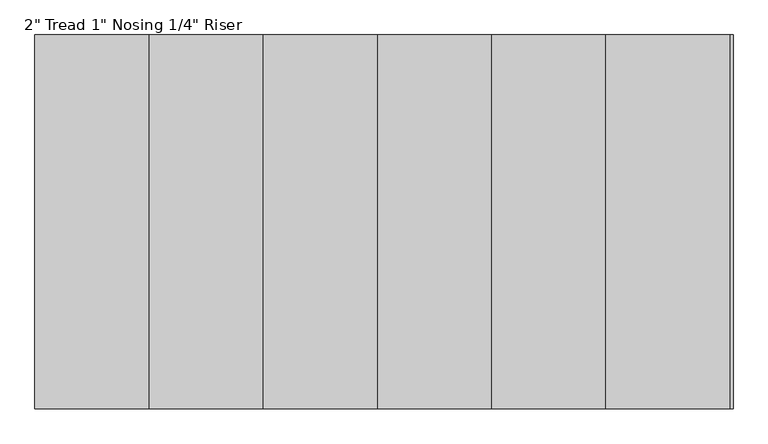
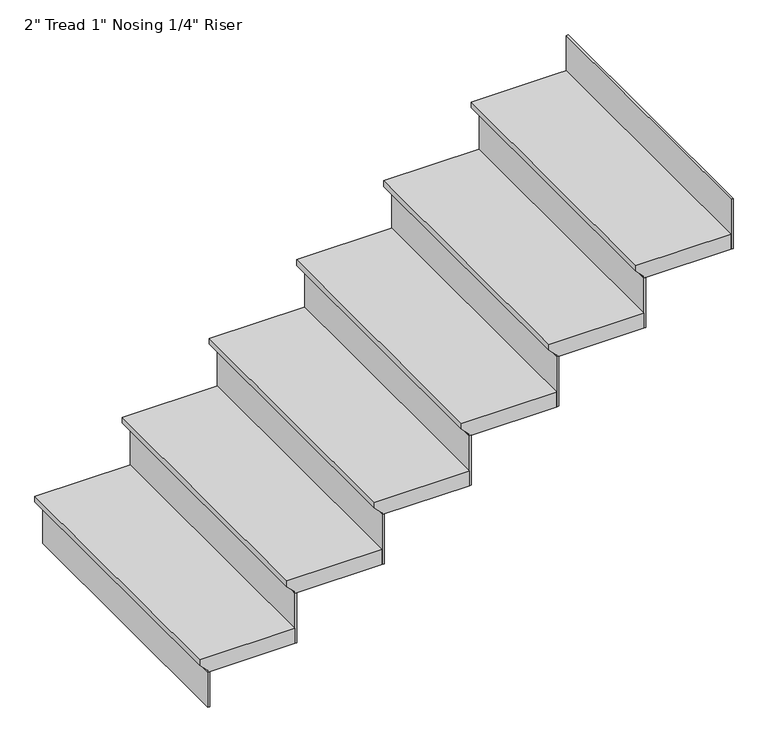
"""IFC4 building model written with IfcOpenShell, lengths in millimetres: stair flight geometry."""

from ifc_helpers import new_model, si_unit, origin, place, context, project, spatial, faceted_brep, source, transform, mapped, element, save


def stair_flight_dd3871da(model_context):
    return source(origin(), model_context, "Body", "Brep", [
        faceted_brep([(-2479.5608498, 3565.3115866, 150.2833333), (-2479.5608498, 3565.3115866, 169.3333333), (-2479.5608498, 4479.7115866, 169.3333333), (-2479.5608498, 4479.7115866, 150.2833333), (-2454.1608498, 3565.3115866, 124.8833333), (-2454.1608498, 4479.7115866, 124.8833333), (-2174.7608498, 3565.3115866, 169.3333333), (-2174.7608498, 4479.7115866, 169.3333333), (-2454.1608498, 4479.7115866, 118.5333333), (-2174.7608498, 4479.7115866, 118.5333333), (-2174.7608498, 3565.3115866, 118.5333333), (-2454.1608498, 3565.3115866, 118.5333333)], [[[0, 1, 2, 3]], [[4, 0, 3, 5]], [[2, 1, 6, 7]], [[8, 9, 10, 11]], [[2, 7, 9, 8, 5, 3]], [[8, 11, 4, 5]], [[6, 1, 0, 4, 11, 10]], [[7, 6, 10, 9]]]),
        faceted_brep([(-2454.1608498, 3565.3115866, 118.5333333), (-2454.1608498, 3565.3115866, 0.0), (-2447.8108498, 3565.3115866, 0.0), (-2447.8108498, 3565.3115866, 118.5333333), (-2454.1608498, 4479.7115866, 118.5333333), (-2447.8108498, 4479.7115866, 118.5333333), (-2447.8108498, 4479.7115866, 0.0), (-2454.1608498, 4479.7115866, 0.0)], [[[0, 1, 2, 3]], [[4, 5, 6, 7]], [[1, 0, 4, 7]], [[2, 1, 7, 6]], [[3, 2, 6, 5]], [[0, 3, 5, 4]]]),
        faceted_brep([(-2174.7608498, 3565.3115866, 287.8666667), (-2174.7608498, 3565.3115866, 118.5333333), (-2168.4108498, 3565.3115866, 118.5333333), (-2168.4108498, 3565.3115866, 287.8666667), (-2174.7608498, 4479.7115866, 287.8666667), (-2168.4108498, 4479.7115866, 287.8666667), (-2168.4108498, 4479.7115866, 118.5333333), (-2174.7608498, 4479.7115866, 118.5333333)], [[[0, 1, 2, 3]], [[4, 5, 6, 7]], [[1, 0, 4, 7]], [[2, 1, 7, 6]], [[3, 2, 6, 5]], [[0, 3, 5, 4]]]),
        faceted_brep([(-2200.1608498, 4479.7115866, 338.6666667), (-2200.1608498, 3565.3115866, 338.6666667), (-1895.3608498, 3565.3115866, 338.6666667), (-1895.3608498, 4479.7115866, 338.6666667), (-2174.7608498, 4479.7115866, 287.8666667), (-1895.3608498, 4479.7115866, 287.8666667), (-1895.3608498, 3565.3115866, 287.8666667), (-2174.7608498, 3565.3115866, 287.8666667), (-2174.7608498, 4479.7115866, 294.2166667), (-2200.1608498, 4479.7115866, 319.6166667), (-2174.7608498, 3565.3115866, 294.2166667), (-2200.1608498, 3565.3115866, 319.6166667)], [[[0, 1, 2, 3]], [[4, 5, 6, 7]], [[0, 3, 5, 4, 8, 9]], [[4, 7, 10, 8]], [[2, 1, 11, 10, 7, 6]], [[3, 2, 6, 5]], [[11, 1, 0, 9]], [[10, 11, 9, 8]]]),
        faceted_brep([(-1895.3608498, 3565.3115866, 457.2), (-1895.3608498, 3565.3115866, 287.8666667), (-1889.0108498, 3565.3115866, 287.8666667), (-1889.0108498, 3565.3115866, 457.2), (-1895.3608498, 4479.7115866, 457.2), (-1889.0108498, 4479.7115866, 457.2), (-1889.0108498, 4479.7115866, 287.8666667), (-1895.3608498, 4479.7115866, 287.8666667)], [[[0, 1, 2, 3]], [[4, 5, 6, 7]], [[1, 0, 4, 7]], [[2, 1, 7, 6]], [[3, 2, 6, 5]], [[0, 3, 5, 4]]]),
        faceted_brep([(-1920.7608498, 4479.7115866, 508.0), (-1920.7608498, 3565.3115866, 508.0), (-1615.9608498, 3565.3115866, 508.0), (-1615.9608498, 4479.7115866, 508.0), (-1895.3608498, 4479.7115866, 457.2), (-1615.9608498, 4479.7115866, 457.2), (-1615.9608498, 3565.3115866, 457.2), (-1895.3608498, 3565.3115866, 457.2), (-1895.3608498, 4479.7115866, 463.55), (-1920.7608498, 4479.7115866, 488.95), (-1895.3608498, 3565.3115866, 463.55), (-1920.7608498, 3565.3115866, 488.95)], [[[0, 1, 2, 3]], [[4, 5, 6, 7]], [[0, 3, 5, 4, 8, 9]], [[4, 7, 10, 8]], [[2, 1, 11, 10, 7, 6]], [[3, 2, 6, 5]], [[11, 1, 0, 9]], [[10, 11, 9, 8]]]),
        faceted_brep([(-1615.9608498, 3565.3115866, 626.5333333), (-1615.9608498, 3565.3115866, 457.2), (-1609.6108498, 3565.3115866, 457.2), (-1609.6108498, 3565.3115866, 626.5333333), (-1615.9608498, 4479.7115866, 626.5333333), (-1609.6108498, 4479.7115866, 626.5333333), (-1609.6108498, 4479.7115866, 457.2), (-1615.9608498, 4479.7115866, 457.2)], [[[0, 1, 2, 3]], [[4, 5, 6, 7]], [[1, 0, 4, 7]], [[2, 1, 7, 6]], [[3, 2, 6, 5]], [[0, 3, 5, 4]]]),
        faceted_brep([(-1641.3608498, 4479.7115866, 677.3333333), (-1641.3608498, 3565.3115866, 677.3333333), (-1336.5608498, 3565.3115866, 677.3333333), (-1336.5608498, 4479.7115866, 677.3333333), (-1615.9608498, 4479.7115866, 626.5333333), (-1336.5608498, 4479.7115866, 626.5333333), (-1336.5608498, 3565.3115866, 626.5333333), (-1615.9608498, 3565.3115866, 626.5333333), (-1615.9608498, 4479.7115866, 632.8833333), (-1641.3608498, 4479.7115866, 658.2833333), (-1615.9608498, 3565.3115866, 632.8833333), (-1641.3608498, 3565.3115866, 658.2833333)], [[[0, 1, 2, 3]], [[4, 5, 6, 7]], [[0, 3, 5, 4, 8, 9]], [[4, 7, 10, 8]], [[2, 1, 11, 10, 7, 6]], [[3, 2, 6, 5]], [[11, 1, 0, 9]], [[10, 11, 9, 8]]]),
        faceted_brep([(-1336.5608498, 3565.3115866, 795.8666667), (-1336.5608498, 3565.3115866, 626.5333333), (-1330.2108498, 3565.3115866, 626.5333333), (-1330.2108498, 3565.3115866, 795.8666667), (-1336.5608498, 4479.7115866, 795.8666667), (-1330.2108498, 4479.7115866, 795.8666667), (-1330.2108498, 4479.7115866, 626.5333333), (-1336.5608498, 4479.7115866, 626.5333333)], [[[0, 1, 2, 3]], [[4, 5, 6, 7]], [[1, 0, 4, 7]], [[2, 1, 7, 6]], [[3, 2, 6, 5]], [[0, 3, 5, 4]]]),
        faceted_brep([(-1361.9608498, 4479.7115866, 846.6666667), (-1361.9608498, 3565.3115866, 846.6666667), (-1057.1608498, 3565.3115866, 846.6666667), (-1057.1608498, 4479.7115866, 846.6666667), (-1336.5608498, 4479.7115866, 795.8666667), (-1057.1608498, 4479.7115866, 795.8666667), (-1057.1608498, 3565.3115866, 795.8666667), (-1336.5608498, 3565.3115866, 795.8666667), (-1336.5608498, 4479.7115866, 802.2166667), (-1361.9608498, 4479.7115866, 827.6166667), (-1336.5608498, 3565.3115866, 802.2166667), (-1361.9608498, 3565.3115866, 827.6166667)], [[[0, 1, 2, 3]], [[4, 5, 6, 7]], [[0, 3, 5, 4, 8, 9]], [[4, 7, 10, 8]], [[2, 1, 11, 10, 7, 6]], [[3, 2, 6, 5]], [[11, 1, 0, 9]], [[10, 11, 9, 8]]]),
        faceted_brep([(-777.7608498, 3565.3115866, 1134.5333333), (-777.7608498, 3565.3115866, 965.2), (-771.4108498, 3565.3115866, 965.2), (-771.4108498, 3565.3115866, 1134.5333333), (-777.7608498, 4479.7115866, 1134.5333333), (-771.4108498, 4479.7115866, 1134.5333333), (-771.4108498, 4479.7115866, 965.2), (-777.7608498, 4479.7115866, 965.2)], [[[0, 1, 2, 3]], [[4, 5, 6, 7]], [[1, 0, 4, 7]], [[2, 1, 7, 6]], [[3, 2, 6, 5]], [[0, 3, 5, 4]]]),
        faceted_brep([(-1057.1608498, 3565.3115866, 965.2), (-1057.1608498, 3565.3115866, 795.8666667), (-1050.8108498, 3565.3115866, 795.8666667), (-1050.8108498, 3565.3115866, 965.2), (-1057.1608498, 4479.7115866, 965.2), (-1050.8108498, 4479.7115866, 965.2), (-1050.8108498, 4479.7115866, 795.8666667), (-1057.1608498, 4479.7115866, 795.8666667)], [[[0, 1, 2, 3]], [[4, 5, 6, 7]], [[1, 0, 4, 7]], [[2, 1, 7, 6]], [[3, 2, 6, 5]], [[0, 3, 5, 4]]]),
        faceted_brep([(-777.7608498, 4479.7115866, 1016.0), (-803.1608498, 4479.7115866, 1016.0), (-1082.5608498, 4479.7115866, 1016.0), (-1082.5608498, 3565.3115866, 1016.0), (-777.7608498, 3565.3115866, 1016.0), (-803.1608498, 4479.7115866, 965.2), (-777.7608498, 4479.7115866, 965.2), (-777.7608498, 3565.3115866, 965.2), (-1057.1608498, 3565.3115866, 965.2), (-1057.1608498, 4479.7115866, 965.2), (-1057.1608498, 4479.7115866, 971.55), (-1082.5608498, 4479.7115866, 996.95), (-1057.1608498, 3565.3115866, 971.55), (-1082.5608498, 3565.3115866, 996.95)], [[[0, 1, 2, 3, 4]], [[5, 6, 7, 8, 9]], [[1, 0, 6, 5]], [[2, 1, 5, 9, 10, 11]], [[9, 8, 12, 10]], [[4, 3, 13, 12, 8, 7]], [[0, 4, 7, 6]], [[13, 3, 2, 11]], [[12, 13, 11, 10]]]),
    ])


if __name__ == "__main__":
    model = new_model("IFC4")
    model_context = context("Model", 3, world=origin())
    ifc_project = project(units=[si_unit("LENGTHUNIT", "METRE", prefix="MILLI")], contexts=[model_context])
    site = spatial("IfcSite", under=ifc_project)
    building = spatial("IfcBuilding", under=site)
    placement = place(None, origin())
    stair_flight_shape = stair_flight_dd3871da(model_context)
    element("IfcStairFlight", 1, ObjectType="2\" Tread 1\" Nosing 1/4\" Riser", at=placement, inside=building, context=model_context, shape_type="MappedRepresentation", body=[
        mapped(stair_flight_shape, transform((0.0, 0.0, 0.0), x_axis=(1.0, 0.0, 0.0), y_axis=(0.0, 1.0, 0.0), z_axis=(0.0, 0.0, 1.0))),
    ])
    save(model, "model.ifc")
